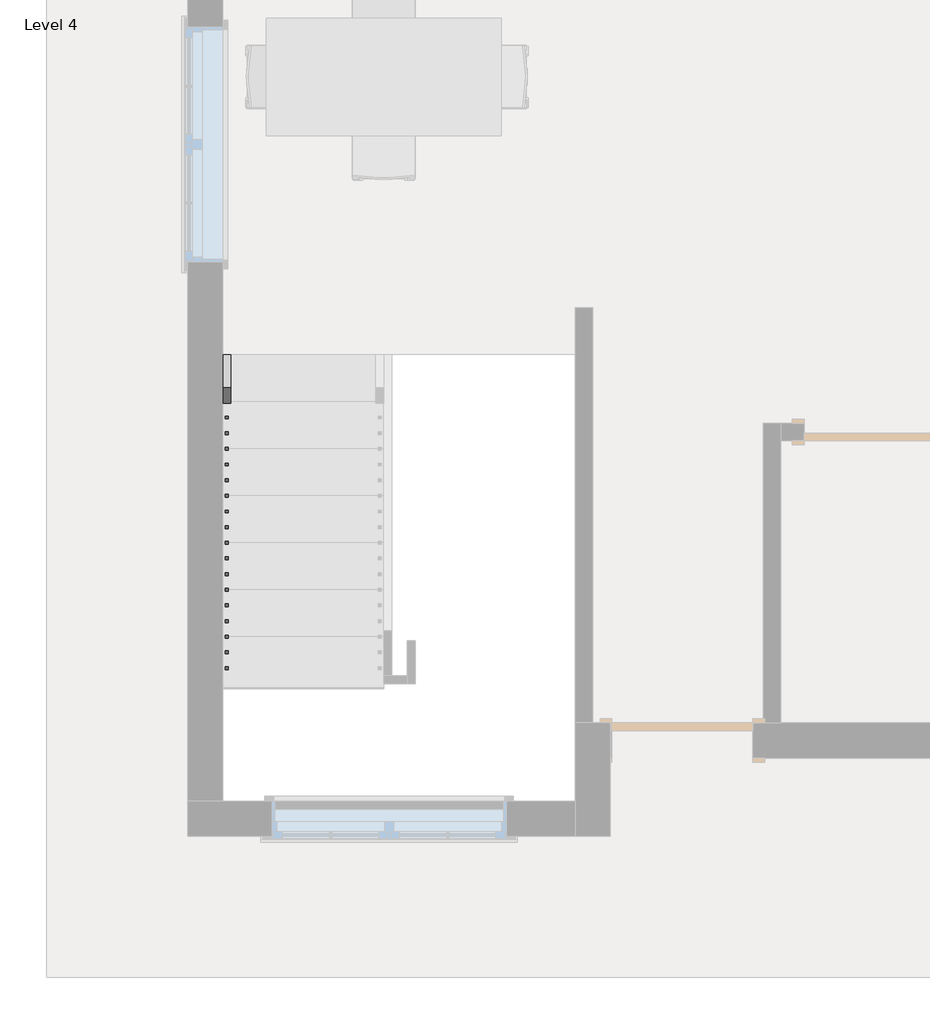
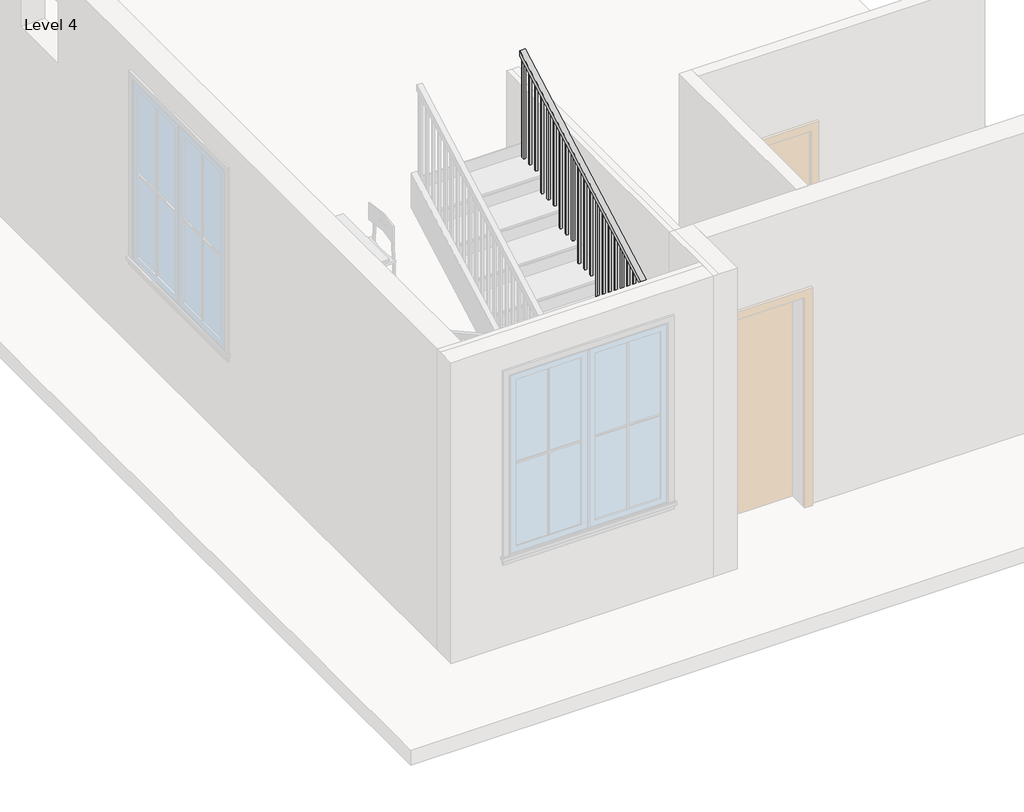
# One storey, part 2 of 3: 1 railing.
"""IFC4 building model written with IfcOpenShell, lengths in millimetres."""

from ifc_helpers import new_model, si_unit, frame, origin, place, context, project, spatial, polyline, outline, extrude, faceted_brep, element, save

model = new_model("IFC4")

# Units and contexts
model_context = context("Model", 3, world=origin())
ifc_project = project(units=[si_unit("LENGTHUNIT", "METRE", prefix="MILLI")], contexts=[model_context])

# Site, building, storey
site = spatial("IfcSite", under=ifc_project)
building = spatial("IfcBuilding", under=site)
storey = spatial("IfcBuildingStorey", under=building, Name="Level 4", Elevation=9448.8)

# Railing
placement = place(None, origin())
element("IfcRailing", 1, ObjectType="Handrail - Rectangular", at=placement, inside=storey, context=model_context, shape_type="SolidModel", body=[
    faceted_brep([(-4181.480864, -3571.6080018, 10532.5333333), (-4181.480864, -3571.6080018, 10474.420221), (-4232.280864, -3571.6080018, 10474.420221), (-4232.280864, -3571.6080018, 10532.5333333), (-4181.480864, -5705.2080018, 11717.8666667), (-4181.480864, -5718.371604, 11667.0666667), (-4232.280864, -5718.371604, 11667.0666667), (-4232.280864, -5705.2080018, 11717.8666667), (-4181.480864, -6416.4080018, 11717.8666667), (-4181.480864, -6416.4080018, 11667.0666667), (-4232.280864, -6467.2080018, 11667.0666667), (-4232.280864, -6467.2080018, 11717.8666667), (-1997.080864, -6416.4080018, 11717.8666667), (-1997.080864, -6416.4080018, 11667.0666667), (-1946.280864, -6467.2080018, 11667.0666667), (-1946.280864, -6467.2080018, 11717.8666667), (-1997.080864, -5705.2080018, 11717.8666667), (-1997.080864, -5692.0443995, 11667.0666667), (-1946.280864, -5692.0443995, 11667.0666667), (-1946.280864, -5705.2080018, 11717.8666667), (-1997.080864, -3571.6080018, 12903.2), (-1946.280864, -3571.6080018, 12903.2), (-1946.280864, -3571.6080018, 12845.0868876), (-1997.080864, -3571.6080018, 12845.0868876)], [[[0, 1, 2, 3]], [[1, 0, 4, 5]], [[2, 1, 5, 6]], [[3, 2, 6, 7]], [[0, 3, 7, 4]], [[5, 4, 8, 9]], [[6, 5, 9, 10]], [[7, 6, 10, 11]], [[4, 7, 11, 8]], [[9, 8, 12, 13]], [[10, 9, 13, 14]], [[11, 10, 14, 15]], [[8, 11, 15, 12]], [[13, 12, 16, 17]], [[14, 13, 17, 18]], [[15, 14, 18, 19]], [[12, 15, 19, 16]], [[20, 21, 22, 23]], [[17, 16, 20, 23]], [[18, 17, 23, 22]], [[19, 18, 22, 21]], [[16, 19, 21, 20]]]),
    extrude(outline(polyline([(-3606.5330018, 12825.6841099), (-3587.4830018, 12836.2674432), (-3587.4830018, 11819.4666667), (-3606.5330018, 11819.4666667), (-3606.5330018, 12825.6841099)])), frame((-1981.205864, 0.0, 0.0), z_axis=(1.0, 0.0, 0.0), x_axis=(0.0, 1.0, 0.0)), (0.0, 0.0, 1.0), 19.05),
    extrude(outline(polyline([(-3708.1330018, 12769.2396654), (-3689.0830018, 12779.8229988), (-3689.0830018, 11819.4666667), (-3708.1330018, 11819.4666667), (-3708.1330018, 12769.2396654)])), frame((-1981.205864, 0.0, 0.0), z_axis=(1.0, 0.0, 0.0), x_axis=(0.0, 1.0, 0.0)), (0.0, 0.0, 1.0), 19.05),
    extrude(outline(polyline([(-3809.7330018, 12712.795221), (-3790.6830018, 12723.3785543), (-3790.6830018, 11819.4666667), (-3809.7330018, 11819.4666667), (-3809.7330018, 12712.795221)])), frame((-1981.205864, 0.0, 0.0), z_axis=(1.0, 0.0, 0.0), x_axis=(0.0, 1.0, 0.0)), (0.0, 0.0, 1.0), 19.05),
    extrude(outline(polyline([(-3911.3330018, 12656.3507765), (-3892.2830018, 12666.9341099), (-3892.2830018, 11650.1333333), (-3911.3330018, 11650.1333333), (-3911.3330018, 12656.3507765)])), frame((-1981.205864, 0.0, 0.0), z_axis=(1.0, 0.0, 0.0), x_axis=(0.0, 1.0, 0.0)), (0.0, 0.0, 1.0), 19.05),
    extrude(outline(polyline([(-4012.9330018, 12599.9063321), (-3993.8830018, 12610.4896654), (-3993.8830018, 11650.1333333), (-4012.9330018, 11650.1333333), (-4012.9330018, 12599.9063321)])), frame((-1981.205864, 0.0, 0.0), z_axis=(1.0, 0.0, 0.0), x_axis=(0.0, 1.0, 0.0)), (0.0, 0.0, 1.0), 19.05),
    extrude(outline(polyline([(-4114.5330018, 12543.4618876), (-4095.4830018, 12554.045221), (-4095.4830018, 11650.1333333), (-4114.5330018, 11650.1333333), (-4114.5330018, 12543.4618876)])), frame((-1981.205864, 0.0, 0.0), z_axis=(1.0, 0.0, 0.0), x_axis=(0.0, 1.0, 0.0)), (0.0, 0.0, 1.0), 19.05),
    extrude(outline(polyline([(-4216.1330018, 12487.0174432), (-4197.0830018, 12497.6007765), (-4197.0830018, 11480.8), (-4216.1330018, 11480.8), (-4216.1330018, 12487.0174432)])), frame((-1981.205864, 0.0, 0.0), z_axis=(1.0, 0.0, 0.0), x_axis=(0.0, 1.0, 0.0)), (0.0, 0.0, 1.0), 19.05),
    extrude(outline(polyline([(-4317.7330018, 12430.5729988), (-4298.6830018, 12441.1563321), (-4298.6830018, 11480.8), (-4317.7330018, 11480.8), (-4317.7330018, 12430.5729988)])), frame((-1981.205864, 0.0, 0.0), z_axis=(1.0, 0.0, 0.0), x_axis=(0.0, 1.0, 0.0)), (0.0, 0.0, 1.0), 19.05),
    extrude(outline(polyline([(-4419.3330018, 12374.1285543), (-4400.2830018, 12384.7118876), (-4400.2830018, 11480.8), (-4419.3330018, 11480.8), (-4419.3330018, 12374.1285543)])), frame((-1981.205864, 0.0, 0.0), z_axis=(1.0, 0.0, 0.0), x_axis=(0.0, 1.0, 0.0)), (0.0, 0.0, 1.0), 19.05),
    extrude(outline(polyline([(-4520.9330018, 12317.6841099), (-4501.8830018, 12328.2674432), (-4501.8830018, 11311.4666667), (-4520.9330018, 11311.4666667), (-4520.9330018, 12317.6841099)])), frame((-1981.205864, 0.0, 0.0), z_axis=(1.0, 0.0, 0.0), x_axis=(0.0, 1.0, 0.0)), (0.0, 0.0, 1.0), 19.05),
    extrude(outline(polyline([(-4622.5330018, 12261.2396654), (-4603.4830018, 12271.8229988), (-4603.4830018, 11311.4666667), (-4622.5330018, 11311.4666667), (-4622.5330018, 12261.2396654)])), frame((-1981.205864, 0.0, 0.0), z_axis=(1.0, 0.0, 0.0), x_axis=(0.0, 1.0, 0.0)), (0.0, 0.0, 1.0), 19.05),
    extrude(outline(polyline([(-4724.1330018, 12204.795221), (-4705.0830018, 12215.3785543), (-4705.0830018, 11311.4666667), (-4724.1330018, 11311.4666667), (-4724.1330018, 12204.795221)])), frame((-1981.205864, 0.0, 0.0), z_axis=(1.0, 0.0, 0.0), x_axis=(0.0, 1.0, 0.0)), (0.0, 0.0, 1.0), 19.05),
    extrude(outline(polyline([(-4825.7330018, 12148.3507765), (-4806.6830018, 12158.9341099), (-4806.6830018, 11142.1333333), (-4825.7330018, 11142.1333333), (-4825.7330018, 12148.3507765)])), frame((-1981.205864, 0.0, 0.0), z_axis=(1.0, 0.0, 0.0), x_axis=(0.0, 1.0, 0.0)), (0.0, 0.0, 1.0), 19.05),
    extrude(outline(polyline([(-4927.3330018, 12091.9063321), (-4908.2830018, 12102.4896654), (-4908.2830018, 11142.1333333), (-4927.3330018, 11142.1333333), (-4927.3330018, 12091.9063321)])), frame((-1981.205864, 0.0, 0.0), z_axis=(1.0, 0.0, 0.0), x_axis=(0.0, 1.0, 0.0)), (0.0, 0.0, 1.0), 19.05),
    extrude(outline(polyline([(-5028.9330018, 12035.4618876), (-5009.8830018, 12046.045221), (-5009.8830018, 11142.1333333), (-5028.9330018, 11142.1333333), (-5028.9330018, 12035.4618876)])), frame((-1981.205864, 0.0, 0.0), z_axis=(1.0, 0.0, 0.0), x_axis=(0.0, 1.0, 0.0)), (0.0, 0.0, 1.0), 19.05),
    extrude(outline(polyline([(-5130.5330018, 11979.0174432), (-5111.4830018, 11989.6007765), (-5111.4830018, 10972.8), (-5130.5330018, 10972.8), (-5130.5330018, 11979.0174432)])), frame((-1981.205864, 0.0, 0.0), z_axis=(1.0, 0.0, 0.0), x_axis=(0.0, 1.0, 0.0)), (0.0, 0.0, 1.0), 19.05),
    extrude(outline(polyline([(-5232.1330018, 11922.5729988), (-5213.0830018, 11933.1563321), (-5213.0830018, 10972.8), (-5232.1330018, 10972.8), (-5232.1330018, 11922.5729988)])), frame((-1981.205864, 0.0, 0.0), z_axis=(1.0, 0.0, 0.0), x_axis=(0.0, 1.0, 0.0)), (0.0, 0.0, 1.0), 19.05),
    extrude(outline(polyline([(-5333.7330018, 11866.1285543), (-5314.6830018, 11876.7118876), (-5314.6830018, 10972.8), (-5333.7330018, 10972.8), (-5333.7330018, 11866.1285543)])), frame((-1981.205864, 0.0, 0.0), z_axis=(1.0, 0.0, 0.0), x_axis=(0.0, 1.0, 0.0)), (0.0, 0.0, 1.0), 19.05),
    extrude(outline(polyline([(-5435.3330018, 11809.6841099), (-5416.2830018, 11820.2674432), (-5416.2830018, 10803.4666667), (-5435.3330018, 10803.4666667), (-5435.3330018, 11809.6841099)])), frame((-1981.205864, 0.0, 0.0), z_axis=(1.0, 0.0, 0.0), x_axis=(0.0, 1.0, 0.0)), (0.0, 0.0, 1.0), 19.05),
    extrude(outline(polyline([(-5536.9330018, 11753.2396654), (-5517.8830018, 11763.8229988), (-5517.8830018, 10803.4666667), (-5536.9330018, 10803.4666667), (-5536.9330018, 11753.2396654)])), frame((-1981.205864, 0.0, 0.0), z_axis=(1.0, 0.0, 0.0), x_axis=(0.0, 1.0, 0.0)), (0.0, 0.0, 1.0), 19.05),
    extrude(outline(polyline([(-5638.5330018, 11696.795221), (-5619.4830018, 11707.3785543), (-5619.4830018, 10803.4666667), (-5638.5330018, 10803.4666667), (-5638.5330018, 11696.795221)])), frame((-1981.205864, 0.0, 0.0), z_axis=(1.0, 0.0, 0.0), x_axis=(0.0, 1.0, 0.0)), (0.0, 0.0, 1.0), 19.05),
    extrude(outline(polyline([(-1962.155864, -5740.1330018), (-1981.205864, -5740.1330018), (-1981.205864, -5721.0830018), (-1962.155864, -5721.0830018), (-1962.155864, -5740.1330018)])), frame((0.0, 0.0, 10803.4666667), z_axis=(0.0, 0.0, 1.0), x_axis=(1.0, 0.0, 0.0)), (0.0, 0.0, 1.0), 863.6),
    extrude(outline(polyline([(-1962.155864, -5841.7330018), (-1981.205864, -5841.7330018), (-1981.205864, -5822.6830018), (-1962.155864, -5822.6830018), (-1962.155864, -5841.7330018)])), frame((0.0, 0.0, 10803.4666667), z_axis=(0.0, 0.0, 1.0), x_axis=(1.0, 0.0, 0.0)), (0.0, 0.0, 1.0), 863.6),
    extrude(outline(polyline([(-1962.155864, -5943.3330018), (-1981.205864, -5943.3330018), (-1981.205864, -5924.2830018), (-1962.155864, -5924.2830018), (-1962.155864, -5943.3330018)])), frame((0.0, 0.0, 10803.4666667), z_axis=(0.0, 0.0, 1.0), x_axis=(1.0, 0.0, 0.0)), (0.0, 0.0, 1.0), 863.6),
    extrude(outline(polyline([(-1962.155864, -6044.9330018), (-1981.205864, -6044.9330018), (-1981.205864, -6025.8830018), (-1962.155864, -6025.8830018), (-1962.155864, -6044.9330018)])), frame((0.0, 0.0, 10803.4666667), z_axis=(0.0, 0.0, 1.0), x_axis=(1.0, 0.0, 0.0)), (0.0, 0.0, 1.0), 863.6),
    extrude(outline(polyline([(-1962.155864, -6146.5330018), (-1981.205864, -6146.5330018), (-1981.205864, -6127.4830018), (-1962.155864, -6127.4830018), (-1962.155864, -6146.5330018)])), frame((0.0, 0.0, 10803.4666667), z_axis=(0.0, 0.0, 1.0), x_axis=(1.0, 0.0, 0.0)), (0.0, 0.0, 1.0), 863.6),
    extrude(outline(polyline([(-1962.155864, -6248.1330018), (-1981.205864, -6248.1330018), (-1981.205864, -6229.0830018), (-1962.155864, -6229.0830018), (-1962.155864, -6248.1330018)])), frame((0.0, 0.0, 10803.4666667), z_axis=(0.0, 0.0, 1.0), x_axis=(1.0, 0.0, 0.0)), (0.0, 0.0, 1.0), 863.6),
    extrude(outline(polyline([(-1962.155864, -6349.7330018), (-1981.205864, -6349.7330018), (-1981.205864, -6330.6830018), (-1962.155864, -6330.6830018), (-1962.155864, -6349.7330018)])), frame((0.0, 0.0, 10803.4666667), z_axis=(0.0, 0.0, 1.0), x_axis=(1.0, 0.0, 0.0)), (0.0, 0.0, 1.0), 863.6),
    extrude(outline(polyline([(-2082.805864, -6451.3330018), (-2082.805864, -6432.2830018), (-2063.755864, -6432.2830018), (-2063.755864, -6451.3330018), (-2082.805864, -6451.3330018)])), frame((0.0, 0.0, 10803.4666667), z_axis=(0.0, 0.0, 1.0), x_axis=(1.0, 0.0, 0.0)), (0.0, 0.0, 1.0), 863.6),
    extrude(outline(polyline([(-2184.405864, -6451.3330018), (-2184.405864, -6432.2830018), (-2165.355864, -6432.2830018), (-2165.355864, -6451.3330018), (-2184.405864, -6451.3330018)])), frame((0.0, 0.0, 10803.4666667), z_axis=(0.0, 0.0, 1.0), x_axis=(1.0, 0.0, 0.0)), (0.0, 0.0, 1.0), 863.6),
    extrude(outline(polyline([(-2286.005864, -6451.3330018), (-2286.005864, -6432.2830018), (-2266.955864, -6432.2830018), (-2266.955864, -6451.3330018), (-2286.005864, -6451.3330018)])), frame((0.0, 0.0, 10803.4666667), z_axis=(0.0, 0.0, 1.0), x_axis=(1.0, 0.0, 0.0)), (0.0, 0.0, 1.0), 863.6),
    extrude(outline(polyline([(-2387.605864, -6451.3330018), (-2387.605864, -6432.2830018), (-2368.555864, -6432.2830018), (-2368.555864, -6451.3330018), (-2387.605864, -6451.3330018)])), frame((0.0, 0.0, 10803.4666667), z_axis=(0.0, 0.0, 1.0), x_axis=(1.0, 0.0, 0.0)), (0.0, 0.0, 1.0), 863.6),
    extrude(outline(polyline([(-2489.205864, -6451.3330018), (-2489.205864, -6432.2830018), (-2470.155864, -6432.2830018), (-2470.155864, -6451.3330018), (-2489.205864, -6451.3330018)])), frame((0.0, 0.0, 10803.4666667), z_axis=(0.0, 0.0, 1.0), x_axis=(1.0, 0.0, 0.0)), (0.0, 0.0, 1.0), 863.6),
    extrude(outline(polyline([(-2590.805864, -6451.3330018), (-2590.805864, -6432.2830018), (-2571.755864, -6432.2830018), (-2571.755864, -6451.3330018), (-2590.805864, -6451.3330018)])), frame((0.0, 0.0, 10803.4666667), z_axis=(0.0, 0.0, 1.0), x_axis=(1.0, 0.0, 0.0)), (0.0, 0.0, 1.0), 863.6),
    extrude(outline(polyline([(-2692.405864, -6451.3330018), (-2692.405864, -6432.2830018), (-2673.355864, -6432.2830018), (-2673.355864, -6451.3330018), (-2692.405864, -6451.3330018)])), frame((0.0, 0.0, 10803.4666667), z_axis=(0.0, 0.0, 1.0), x_axis=(1.0, 0.0, 0.0)), (0.0, 0.0, 1.0), 863.6),
    extrude(outline(polyline([(-2794.005864, -6451.3330018), (-2794.005864, -6432.2830018), (-2774.955864, -6432.2830018), (-2774.955864, -6451.3330018), (-2794.005864, -6451.3330018)])), frame((0.0, 0.0, 10803.4666667), z_axis=(0.0, 0.0, 1.0), x_axis=(1.0, 0.0, 0.0)), (0.0, 0.0, 1.0), 863.6),
    extrude(outline(polyline([(-2895.605864, -6451.3330018), (-2895.605864, -6432.2830018), (-2876.555864, -6432.2830018), (-2876.555864, -6451.3330018), (-2895.605864, -6451.3330018)])), frame((0.0, 0.0, 10803.4666667), z_axis=(0.0, 0.0, 1.0), x_axis=(1.0, 0.0, 0.0)), (0.0, 0.0, 1.0), 863.6),
    extrude(outline(polyline([(-2997.205864, -6451.3330018), (-2997.205864, -6432.2830018), (-2978.155864, -6432.2830018), (-2978.155864, -6451.3330018), (-2997.205864, -6451.3330018)])), frame((0.0, 0.0, 10803.4666667), z_axis=(0.0, 0.0, 1.0), x_axis=(1.0, 0.0, 0.0)), (0.0, 0.0, 1.0), 863.6),
    extrude(outline(polyline([(-3098.805864, -6451.3330018), (-3098.805864, -6432.2830018), (-3079.755864, -6432.2830018), (-3079.755864, -6451.3330018), (-3098.805864, -6451.3330018)])), frame((0.0, 0.0, 10803.4666667), z_axis=(0.0, 0.0, 1.0), x_axis=(1.0, 0.0, 0.0)), (0.0, 0.0, 1.0), 863.6),
    extrude(outline(polyline([(-3200.405864, -6451.3330018), (-3200.405864, -6432.2830018), (-3181.355864, -6432.2830018), (-3181.355864, -6451.3330018), (-3200.405864, -6451.3330018)])), frame((0.0, 0.0, 10803.4666667), z_axis=(0.0, 0.0, 1.0), x_axis=(1.0, 0.0, 0.0)), (0.0, 0.0, 1.0), 863.6),
    extrude(outline(polyline([(-3302.005864, -6451.3330018), (-3302.005864, -6432.2830018), (-3282.955864, -6432.2830018), (-3282.955864, -6451.3330018), (-3302.005864, -6451.3330018)])), frame((0.0, 0.0, 10803.4666667), z_axis=(0.0, 0.0, 1.0), x_axis=(1.0, 0.0, 0.0)), (0.0, 0.0, 1.0), 863.6),
    extrude(outline(polyline([(-3403.605864, -6451.3330018), (-3403.605864, -6432.2830018), (-3384.555864, -6432.2830018), (-3384.555864, -6451.3330018), (-3403.605864, -6451.3330018)])), frame((0.0, 0.0, 10803.4666667), z_axis=(0.0, 0.0, 1.0), x_axis=(1.0, 0.0, 0.0)), (0.0, 0.0, 1.0), 863.6),
    extrude(outline(polyline([(-3505.205864, -6451.3330018), (-3505.205864, -6432.2830018), (-3486.155864, -6432.2830018), (-3486.155864, -6451.3330018), (-3505.205864, -6451.3330018)])), frame((0.0, 0.0, 10803.4666667), z_axis=(0.0, 0.0, 1.0), x_axis=(1.0, 0.0, 0.0)), (0.0, 0.0, 1.0), 863.6),
    extrude(outline(polyline([(-3606.805864, -6451.3330018), (-3606.805864, -6432.2830018), (-3587.755864, -6432.2830018), (-3587.755864, -6451.3330018), (-3606.805864, -6451.3330018)])), frame((0.0, 0.0, 10803.4666667), z_axis=(0.0, 0.0, 1.0), x_axis=(1.0, 0.0, 0.0)), (0.0, 0.0, 1.0), 863.6),
    extrude(outline(polyline([(-3708.405864, -6451.3330018), (-3708.405864, -6432.2830018), (-3689.355864, -6432.2830018), (-3689.355864, -6451.3330018), (-3708.405864, -6451.3330018)])), frame((0.0, 0.0, 10803.4666667), z_axis=(0.0, 0.0, 1.0), x_axis=(1.0, 0.0, 0.0)), (0.0, 0.0, 1.0), 863.6),
    extrude(outline(polyline([(-3810.005864, -6451.3330018), (-3810.005864, -6432.2830018), (-3790.955864, -6432.2830018), (-3790.955864, -6451.3330018), (-3810.005864, -6451.3330018)])), frame((0.0, 0.0, 10803.4666667), z_axis=(0.0, 0.0, 1.0), x_axis=(1.0, 0.0, 0.0)), (0.0, 0.0, 1.0), 863.6),
    extrude(outline(polyline([(-3911.605864, -6451.3330018), (-3911.605864, -6432.2830018), (-3892.555864, -6432.2830018), (-3892.555864, -6451.3330018), (-3911.605864, -6451.3330018)])), frame((0.0, 0.0, 10803.4666667), z_axis=(0.0, 0.0, 1.0), x_axis=(1.0, 0.0, 0.0)), (0.0, 0.0, 1.0), 863.6),
    extrude(outline(polyline([(-4013.205864, -6451.3330018), (-4013.205864, -6432.2830018), (-3994.155864, -6432.2830018), (-3994.155864, -6451.3330018), (-4013.205864, -6451.3330018)])), frame((0.0, 0.0, 10803.4666667), z_axis=(0.0, 0.0, 1.0), x_axis=(1.0, 0.0, 0.0)), (0.0, 0.0, 1.0), 863.6),
    extrude(outline(polyline([(-4114.805864, -6451.3330018), (-4114.805864, -6432.2830018), (-4095.755864, -6432.2830018), (-4095.755864, -6451.3330018), (-4114.805864, -6451.3330018)])), frame((0.0, 0.0, 10803.4666667), z_axis=(0.0, 0.0, 1.0), x_axis=(1.0, 0.0, 0.0)), (0.0, 0.0, 1.0), 863.6),
    extrude(outline(polyline([(-4216.405864, -6406.8830018), (-4197.355864, -6406.8830018), (-4197.355864, -6425.9330018), (-4216.405864, -6425.9330018), (-4216.405864, -6406.8830018)])), frame((0.0, 0.0, 10803.4666667), z_axis=(0.0, 0.0, 1.0), x_axis=(1.0, 0.0, 0.0)), (0.0, 0.0, 1.0), 863.6),
    extrude(outline(polyline([(-4216.405864, -6305.2830018), (-4197.355864, -6305.2830018), (-4197.355864, -6324.3330018), (-4216.405864, -6324.3330018), (-4216.405864, -6305.2830018)])), frame((0.0, 0.0, 10803.4666667), z_axis=(0.0, 0.0, 1.0), x_axis=(1.0, 0.0, 0.0)), (0.0, 0.0, 1.0), 863.6),
    extrude(outline(polyline([(-4216.405864, -6203.6830018), (-4197.355864, -6203.6830018), (-4197.355864, -6222.7330018), (-4216.405864, -6222.7330018), (-4216.405864, -6203.6830018)])), frame((0.0, 0.0, 10803.4666667), z_axis=(0.0, 0.0, 1.0), x_axis=(1.0, 0.0, 0.0)), (0.0, 0.0, 1.0), 863.6),
    extrude(outline(polyline([(-4216.405864, -6102.0830018), (-4197.355864, -6102.0830018), (-4197.355864, -6121.1330018), (-4216.405864, -6121.1330018), (-4216.405864, -6102.0830018)])), frame((0.0, 0.0, 10803.4666667), z_axis=(0.0, 0.0, 1.0), x_axis=(1.0, 0.0, 0.0)), (0.0, 0.0, 1.0), 863.6),
    extrude(outline(polyline([(-4216.405864, -6000.4830018), (-4197.355864, -6000.4830018), (-4197.355864, -6019.5330018), (-4216.405864, -6019.5330018), (-4216.405864, -6000.4830018)])), frame((0.0, 0.0, 10803.4666667), z_axis=(0.0, 0.0, 1.0), x_axis=(1.0, 0.0, 0.0)), (0.0, 0.0, 1.0), 863.6),
    extrude(outline(polyline([(-4216.405864, -5898.8830018), (-4197.355864, -5898.8830018), (-4197.355864, -5917.9330018), (-4216.405864, -5917.9330018), (-4216.405864, -5898.8830018)])), frame((0.0, 0.0, 10803.4666667), z_axis=(0.0, 0.0, 1.0), x_axis=(1.0, 0.0, 0.0)), (0.0, 0.0, 1.0), 863.6),
    extrude(outline(polyline([(-4216.405864, -5797.2830018), (-4197.355864, -5797.2830018), (-4197.355864, -5816.3330018), (-4216.405864, -5816.3330018), (-4216.405864, -5797.2830018)])), frame((0.0, 0.0, 10803.4666667), z_axis=(0.0, 0.0, 1.0), x_axis=(1.0, 0.0, 0.0)), (0.0, 0.0, 1.0), 863.6),
    extrude(outline(polyline([(-5714.7330018, 11665.045221), (-5695.6830018, 11654.4618876), (-5695.6830018, 10803.4666667), (-5714.7330018, 10803.4666667), (-5714.7330018, 11665.045221)])), frame((-4216.405864, 0.0, 0.0), z_axis=(1.0, 0.0, 0.0), x_axis=(0.0, 1.0, 0.0)), (0.0, 0.0, 1.0), 19.05),
    extrude(outline(polyline([(-5613.1330018, 11608.6007765), (-5594.0830018, 11598.0174432), (-5594.0830018, 10634.1333333), (-5613.1330018, 10634.1333333), (-5613.1330018, 11608.6007765)])), frame((-4216.405864, 0.0, 0.0), z_axis=(1.0, 0.0, 0.0), x_axis=(0.0, 1.0, 0.0)), (0.0, 0.0, 1.0), 19.05),
    extrude(outline(polyline([(-5511.5330018, 11552.1563321), (-5492.4830018, 11541.5729988), (-5492.4830018, 10634.1333333), (-5511.5330018, 10634.1333333), (-5511.5330018, 11552.1563321)])), frame((-4216.405864, 0.0, 0.0), z_axis=(1.0, 0.0, 0.0), x_axis=(0.0, 1.0, 0.0)), (0.0, 0.0, 1.0), 19.05),
    extrude(outline(polyline([(-5409.9330018, 11495.7118876), (-5390.8830018, 11485.1285543), (-5390.8830018, 10634.1333333), (-5409.9330018, 10634.1333333), (-5409.9330018, 11495.7118876)])), frame((-4216.405864, 0.0, 0.0), z_axis=(1.0, 0.0, 0.0), x_axis=(0.0, 1.0, 0.0)), (0.0, 0.0, 1.0), 19.05),
    extrude(outline(polyline([(-5308.3330018, 11439.2674432), (-5289.2830018, 11428.6841099), (-5289.2830018, 10464.8), (-5308.3330018, 10464.8), (-5308.3330018, 11439.2674432)])), frame((-4216.405864, 0.0, 0.0), z_axis=(1.0, 0.0, 0.0), x_axis=(0.0, 1.0, 0.0)), (0.0, 0.0, 1.0), 19.05),
    extrude(outline(polyline([(-5206.7330018, 11382.8229988), (-5187.6830018, 11372.2396654), (-5187.6830018, 10464.8), (-5206.7330018, 10464.8), (-5206.7330018, 11382.8229988)])), frame((-4216.405864, 0.0, 0.0), z_axis=(1.0, 0.0, 0.0), x_axis=(0.0, 1.0, 0.0)), (0.0, 0.0, 1.0), 19.05),
    extrude(outline(polyline([(-5105.1330018, 11326.3785543), (-5086.0830018, 11315.795221), (-5086.0830018, 10464.8), (-5105.1330018, 10464.8), (-5105.1330018, 11326.3785543)])), frame((-4216.405864, 0.0, 0.0), z_axis=(1.0, 0.0, 0.0), x_axis=(0.0, 1.0, 0.0)), (0.0, 0.0, 1.0), 19.05),
    extrude(outline(polyline([(-5003.5330018, 11269.9341099), (-4984.4830018, 11259.3507765), (-4984.4830018, 10295.4666667), (-5003.5330018, 10295.4666667), (-5003.5330018, 11269.9341099)])), frame((-4216.405864, 0.0, 0.0), z_axis=(1.0, 0.0, 0.0), x_axis=(0.0, 1.0, 0.0)), (0.0, 0.0, 1.0), 19.05),
    extrude(outline(polyline([(-4901.9330018, 11213.4896654), (-4882.8830018, 11202.9063321), (-4882.8830018, 10295.4666667), (-4901.9330018, 10295.4666667), (-4901.9330018, 11213.4896654)])), frame((-4216.405864, 0.0, 0.0), z_axis=(1.0, 0.0, 0.0), x_axis=(0.0, 1.0, 0.0)), (0.0, 0.0, 1.0), 19.05),
    extrude(outline(polyline([(-4800.3330018, 11157.045221), (-4781.2830018, 11146.4618876), (-4781.2830018, 10295.4666667), (-4800.3330018, 10295.4666667), (-4800.3330018, 11157.045221)])), frame((-4216.405864, 0.0, 0.0), z_axis=(1.0, 0.0, 0.0), x_axis=(0.0, 1.0, 0.0)), (0.0, 0.0, 1.0), 19.05),
    extrude(outline(polyline([(-4698.7330018, 11100.6007765), (-4679.6830018, 11090.0174432), (-4679.6830018, 10126.1333333), (-4698.7330018, 10126.1333333), (-4698.7330018, 11100.6007765)])), frame((-4216.405864, 0.0, 0.0), z_axis=(1.0, 0.0, 0.0), x_axis=(0.0, 1.0, 0.0)), (0.0, 0.0, 1.0), 19.05),
    extrude(outline(polyline([(-4597.1330018, 11044.1563321), (-4578.0830018, 11033.5729988), (-4578.0830018, 10126.1333333), (-4597.1330018, 10126.1333333), (-4597.1330018, 11044.1563321)])), frame((-4216.405864, 0.0, 0.0), z_axis=(1.0, 0.0, 0.0), x_axis=(0.0, 1.0, 0.0)), (0.0, 0.0, 1.0), 19.05),
    extrude(outline(polyline([(-4495.5330018, 10987.7118876), (-4476.4830018, 10977.1285543), (-4476.4830018, 10126.1333333), (-4495.5330018, 10126.1333333), (-4495.5330018, 10987.7118876)])), frame((-4216.405864, 0.0, 0.0), z_axis=(1.0, 0.0, 0.0), x_axis=(0.0, 1.0, 0.0)), (0.0, 0.0, 1.0), 19.05),
    extrude(outline(polyline([(-4393.9330018, 10931.2674432), (-4374.8830018, 10920.6841099), (-4374.8830018, 9956.8), (-4393.9330018, 9956.8), (-4393.9330018, 10931.2674432)])), frame((-4216.405864, 0.0, 0.0), z_axis=(1.0, 0.0, 0.0), x_axis=(0.0, 1.0, 0.0)), (0.0, 0.0, 1.0), 19.05),
    extrude(outline(polyline([(-4292.3330018, 10874.8229988), (-4273.2830018, 10864.2396654), (-4273.2830018, 9956.8), (-4292.3330018, 9956.8), (-4292.3330018, 10874.8229988)])), frame((-4216.405864, 0.0, 0.0), z_axis=(1.0, 0.0, 0.0), x_axis=(0.0, 1.0, 0.0)), (0.0, 0.0, 1.0), 19.05),
    extrude(outline(polyline([(-4190.7330018, 10818.3785543), (-4171.6830018, 10807.795221), (-4171.6830018, 9956.8), (-4190.7330018, 9956.8), (-4190.7330018, 10818.3785543)])), frame((-4216.405864, 0.0, 0.0), z_axis=(1.0, 0.0, 0.0), x_axis=(0.0, 1.0, 0.0)), (0.0, 0.0, 1.0), 19.05),
    extrude(outline(polyline([(-4089.1330018, 10761.9341099), (-4070.0830018, 10751.3507765), (-4070.0830018, 9787.4666667), (-4089.1330018, 9787.4666667), (-4089.1330018, 10761.9341099)])), frame((-4216.405864, 0.0, 0.0), z_axis=(1.0, 0.0, 0.0), x_axis=(0.0, 1.0, 0.0)), (0.0, 0.0, 1.0), 19.05),
    extrude(outline(polyline([(-3987.5330018, 10705.4896654), (-3968.4830018, 10694.9063321), (-3968.4830018, 9787.4666667), (-3987.5330018, 9787.4666667), (-3987.5330018, 10705.4896654)])), frame((-4216.405864, 0.0, 0.0), z_axis=(1.0, 0.0, 0.0), x_axis=(0.0, 1.0, 0.0)), (0.0, 0.0, 1.0), 19.05),
    extrude(outline(polyline([(-3885.9330018, 10649.045221), (-3866.8830018, 10638.4618876), (-3866.8830018, 9787.4666667), (-3885.9330018, 9787.4666667), (-3885.9330018, 10649.045221)])), frame((-4216.405864, 0.0, 0.0), z_axis=(1.0, 0.0, 0.0), x_axis=(0.0, 1.0, 0.0)), (0.0, 0.0, 1.0), 19.05),
    extrude(outline(polyline([(-3784.3330018, 10592.6007765), (-3765.2830018, 10582.0174432), (-3765.2830018, 9618.1333333), (-3784.3330018, 9618.1333333), (-3784.3330018, 10592.6007765)])), frame((-4216.405864, 0.0, 0.0), z_axis=(1.0, 0.0, 0.0), x_axis=(0.0, 1.0, 0.0)), (0.0, 0.0, 1.0), 19.05),
    extrude(outline(polyline([(-3682.7330018, 10536.1563321), (-3663.6830018, 10525.5729988), (-3663.6830018, 9618.1333333), (-3682.7330018, 9618.1333333), (-3682.7330018, 10536.1563321)])), frame((-4216.405864, 0.0, 0.0), z_axis=(1.0, 0.0, 0.0), x_axis=(0.0, 1.0, 0.0)), (0.0, 0.0, 1.0), 19.05),
    extrude(outline(polyline([(-1981.205864, -6451.3330018), (-1981.205864, -6432.2830018), (-1962.155864, -6432.2830018), (-1962.155864, -6451.3330018), (-1981.205864, -6451.3330018)])), frame((0.0, 0.0, 10803.4666667), z_axis=(0.0, 0.0, 1.0), x_axis=(1.0, 0.0, 0.0)), (0.0, 0.0, 1.0), 863.6),
    extrude(outline(polyline([(-4216.405864, -6432.2830018), (-4197.355864, -6432.2830018), (-4197.355864, -6451.3330018), (-4216.405864, -6451.3330018), (-4216.405864, -6432.2830018)])), frame((0.0, 0.0, 10803.4666667), z_axis=(0.0, 0.0, 1.0), x_axis=(1.0, 0.0, 0.0)), (0.0, 0.0, 1.0), 863.6),
    extrude(outline(polyline([(-3590.6580018, 12834.5035543), (-3571.6080018, 12845.0868876), (-3571.6080018, 11819.4666667), (-3590.6580018, 11819.4666667), (-3590.6580018, 12834.5035543)])), frame((-1981.205864, 0.0, 0.0), z_axis=(1.0, 0.0, 0.0), x_axis=(0.0, 1.0, 0.0)), (0.0, 0.0, 1.0), 19.05),
    extrude(outline(polyline([(-3590.6580018, 10485.0035543), (-3571.6080018, 10474.420221), (-3571.6080018, 9618.1333333), (-3590.6580018, 9618.1333333), (-3590.6580018, 10485.0035543)])), frame((-4216.405864, 0.0, 0.0), z_axis=(1.0, 0.0, 0.0), x_axis=(0.0, 1.0, 0.0)), (0.0, 0.0, 1.0), 19.05),
])

save(model, "model.ifc")

# Revit data of these elements
# Type "Handrail - Rectangular"
#   Assembly Code = "C2010400"
#   built-in parameter 1008612 = 0.0416667 (stored number, unit not read)
#   built-in parameter 1008611 = 0.0416667 (stored number, unit not read)
#   built-in parameter 1008609 = 0.333333 (stored number, unit not read)
#   built-in parameter 1008604 = 0.166667 (stored number, unit not read)
#   built-in parameter 1008603 = 0.166667 (stored number, unit not read)
#   Railing Height = 3' - 0"
#   built-in parameter 1008630 = 2
#   built-in parameter 1008610 = 2
#   built-in parameter 1008618 = Baluster - Square : 3/4"
# Element 1 (IfcRailing, "Handrail - Rectangular")
#   Phase Created = New Construction
